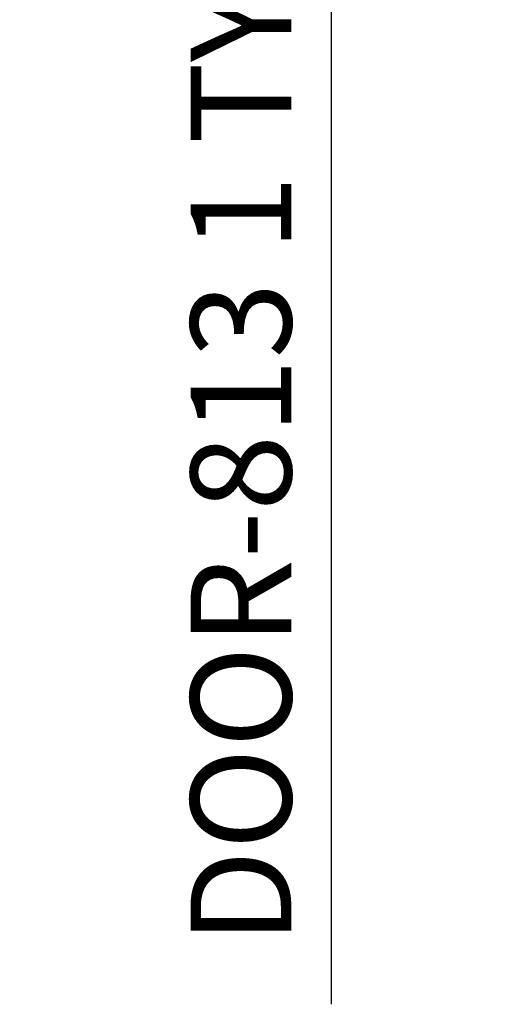
# Model space of a CAD drawing. Units: metres. Extents: x 1246 to 2549, y 2050 to 4184.
# Tile 1 of 6: x 1267 to 1279, y 2050 to 2074. Entities that reach past the tile are written whole.
import ezdxf

# ---------------------------------------------------------------- set-up
doc = ezdxf.new("R2010")
doc.units = ezdxf.units.M
doc.layers.add('A-ANNO-DIMS', color=2, linetype='Continuous', lineweight=18)
doc.styles.get("Standard").update_dxf_attribs({"font": 'arial.ttf'})
doc.dimstyles.new('ISO-25', dxfattribs={"dimtxt": 2.5, "dimasz": 2.5, "dimexe": 1.25, "dimexo": 0.625, "dimtad": 1, "dimtxsty": 'Standard', "dimcen": 2.5, "dimadec": 0, "dimazin": 0, "dimtfac": 1, "dimtmove": 0, "dimatfit": 3, "dimfxl": 1, "dimarcsym": 0})

# ---------------------------------------------------------------- blocks, each defined once
blk = doc.blocks.new('*D7')
at = {"layer": 'A-ANNO-DIMS', "color": 0, "lineweight": -2, "transparency": 16777216}
for p, q in [((1274.837, 2088.031), (1274.837, 2090.531)), ((1274.346, 2085.531), (1273.587, 2085.531)), ((1274.837, 2085.531), (1274.837, 2084.639)), ((1274.346, 2084.639), (1273.587, 2084.639)), ((1274.837, 2082.139), (1274.837, 2049.849))]:
    blk.add_line(p, q, dxfattribs=at)
at = {"layer": 'A-ANNO-DIMS', "color": 0, "transparency": 16777216}
for points in [[(1274.421, 2088.031), (1275.254, 2088.031), (1274.837, 2085.531)], [(1274.421, 2082.139), (1275.254, 2082.139), (1274.837, 2084.639)]]:
    blk.add_solid(points, dxfattribs=at)
at = {"layer": 'Defpoints', "color": 0, "transparency": 16777216}
for p in [(1274.971, 2085.531), (1274.837, 2084.639), (1274.971, 2084.639)]:
    blk.add_point(p, dxfattribs=at)
at = {"layer": 'A-ANNO-DIMS', "color": 0, "transparency": 16777216, "insert": (1272.918, 2064.744), "char_height": 2.5, "attachment_point": 5, "rotation": 90}
blk.add_mtext('DOOR-813 1 TYP.', dxfattribs=at)

msp = doc.modelspace()

# ---------------------------------------------------------------- dimensions: what is measured, and where the dimension line sits
at = {"layer": 'A-ANNO-DIMS'}
dim = msp.add_linear_dim(base=(1274.8373, 2084.6395), p1=(1274.971, 2085.5308), p2=(1274.971, 2084.6395), angle=270, text='DOOR-813 <> TYP.', dimstyle='ISO-25', override={"dimdec": 0, "dimlfac": 1, "dimrnd": 0, "dimzin": 0, "dimdsep": 46, "dimlunit": 2}, dxfattribs=at)
dim.commit()
dim.dimension.update_dxf_attribs({"geometry": '*D7', "text_midpoint": (1272.918, 2064.7444)})

doc.saveas('drawing.dxf')
